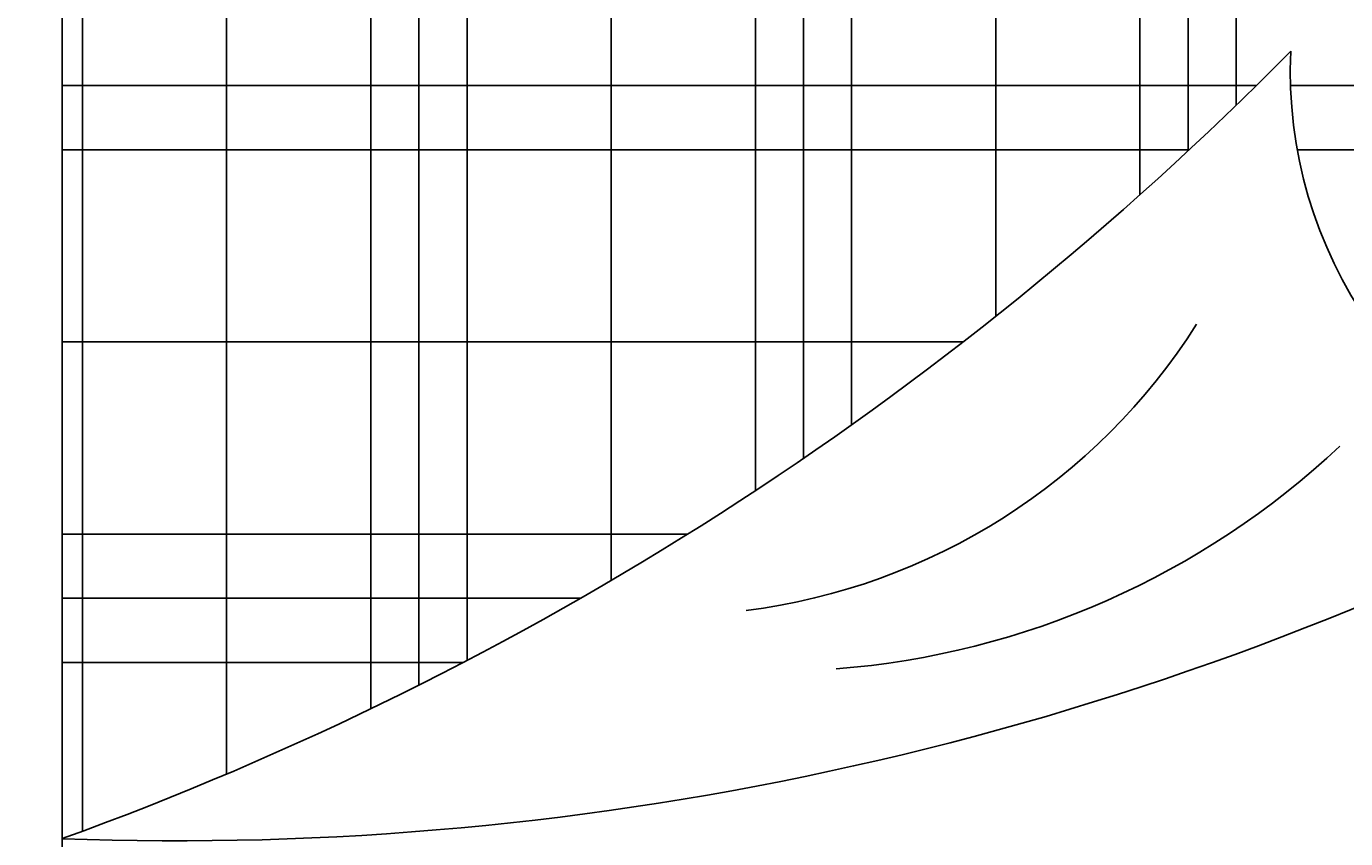
# Model space of a CAD drawing. Units: millimetres. Extents: x 2817 to 5038, y 1110 to 3565.
# Tile 14 of 21: x 2869 to 2917, y 1528 to 1558. Entities that reach past the tile are written whole.
import ezdxf

# ---------------------------------------------------------------- set-up
doc = ezdxf.new("R2010")
doc.units = ezdxf.units.MM
doc.layers.add('A-ANNO-DIMS', color=2, linetype='Continuous', lineweight=18)
doc.layers.add('FURNITURE', color=219, linetype='Continuous', lineweight=18)
doc.layers.add('BLOCK', color=6, linetype='Continuous')
doc.styles.get("Standard").update_dxf_attribs({"font": 'arial.ttf'})
doc.dimstyles.get("Standard").update_dxf_attribs({"dimtxt": 0.18, "dimasz": 0.18, "dimexe": 0.18, "dimexo": 0.0625, "dimgap": 0.09, "dimtad": 0, "dimtih": 1, "dimtoh": 1, "dimdec": 4, "dimzin": 0, "dimdsep": 46, "dimtxsty": 'Standard', "dimcen": 0.09, "dimadec": 0, "dimazin": 0, "dimtfac": 1, "dimtdec": 4, "dimtofl": 0, "dimtmove": 0, "dimatfit": 3, "dimfxl": 1, "dimtolj": 1, "dimtzin": 0, "dimarcsym": 0})

# ---------------------------------------------------------------- blocks, each defined once
blk = doc.blocks.new('*X7')
at = {"color": 0}
for p, q in [((276.598, 451.25), (280.51, 451.25)), ((275.455, 450.625), (280.51, 450.625)), ((274.411, 450), (280.51, 450)), ((271.723, 448.125), (280.51, 448.125)), ((265.51, 446.25), (268.465, 446.25)), ((269.519, 446.25), (280.51, 446.25)), ((265.51, 445.625), (268.531, 445.625)), ((268.866, 445.625), (280.51, 445.625))]:
    blk.add_line(p, q, dxfattribs=at)
blk = doc.blocks.new('*X8')
at = {"color": 0}
for p, q in [((280.312, 439.886), (280.312, 452.896)), ((278.906, 439.482), (278.906, 452.338)), ((277.5, 439.482), (277.5, 451.702)), ((277.031, 439.482), (277.031, 451.471)), ((276.562, 439.482), (276.562, 451.231)), ((275.156, 439.482), (275.156, 450.451)), ((273.75, 439.482), (273.75, 449.576)), ((273.281, 439.482), (273.281, 449.261)), ((272.812, 439.482), (272.812, 448.934)), ((271.406, 439.482), (271.406, 447.876)), ((270, 439.482), (270, 446.689)), ((269.531, 439.482), (269.531, 446.262)), ((269.062, 439.482), (269.062, 445.817))]:
    blk.add_line(p, q, dxfattribs=at)
blk = doc.blocks.new('A$C52E67D0D')
at = {"layer": 'BLOCK'}
blk.add_lwpolyline([(1901, 0), (601, 0, -0.414214), (501, 100), (501, 1700, -0.414214), (601, 1800), (1901, 1800, -0.414214), (2001, 1700), (2001, 100, -0.414214)], format="xyb", close=True, dxfattribs=at)
for centre, radius, start, end in [((1888.6, -1664.5), 3015.3, 87.8642, 117.4001), ((3101, -1685.8), 3227.7, 109.926, 135.3977), ((1308.8, 377.9), 807.6, 94.4436, 133.2788), ((1410.8, 520.2), 610.8, 97.2157, 147.6656), ((371.4, 600.4), 432, 357.3792, 72.5379)]:
    blk.add_arc(centre, radius, start, end, dxfattribs=at)
at = {"layer": 'BLOCK', "xscale": 100, "yscale": 100, "zscale": 100}
for name in ['*X8', '*X7']:
    blk.add_blockref(name, (-26050, -43948.2), dxfattribs=at)
blk = doc.blocks.new('*D38')
at = {"layer": 'A-ANNO-DIMS', "color": 0, "lineweight": -2, "transparency": 16777216}
for p, q in [((3110.177, 1573.436), (2817.308, 1573.436)), ((2817.488, 1573.256), (2817.488, 1523.618)), ((2817.488, 1473.616), (2817.488, 1523.254)), ((3105.677, 1473.436), (2817.308, 1473.436))]:
    blk.add_line(p, q, dxfattribs=at)
for points in [[(2817.458, 1573.256), (2817.518, 1573.256), (2817.488, 1573.436)], [(2817.458, 1473.616), (2817.518, 1473.616), (2817.488, 1473.436)]]:
    blk.add_solid(points, dxfattribs=at)
at = {"layer": 'Defpoints', "color": 0, "lineweight": -2, "transparency": 16777216}
for p in [(2817.488, 1573.436), (3110.239, 1573.436), (3105.739, 1473.436)]:
    blk.add_point(p, dxfattribs=at)
at = {"layer": 'A-ANNO-DIMS', "color": 0, "transparency": 16777216, "insert": (2817.488, 1523.436), "char_height": 0.18, "attachment_point": 5}
blk.add_mtext('\\A1;100', dxfattribs=at)

msp = doc.modelspace()

# ---------------------------------------------------------------- block references
at = {"layer": 'FURNITURE', "xscale": 0.0367705835331598, "yscale": 0.0367705835331598, "zscale": 0.0367705835331598, "rotation": 180}
msp.add_blockref('A$C52E67D0D', (2944.3285, 1578.0385), dxfattribs=at)

# ---------------------------------------------------------------- dimensions: what is measured, and where the dimension line sits
at = {"layer": 'A-ANNO-DIMS'}
dim = msp.add_linear_dim(base=(2817.4881, 1573.4357), p1=(3105.7393, 1473.4357), p2=(3110.2393, 1573.4357), angle=90, dimstyle='Standard', override={"dimdec": 0, "dimlfac": 1, "dimrnd": 0, "dimzin": 0, "dimdsep": 46, "dimlunit": 2}, dxfattribs=at)
dim.commit()
dim.dimension.update_dxf_attribs({"geometry": '*D38', "text_midpoint": (2817.4881, 1523.4357)})

doc.saveas('drawing.dxf')
